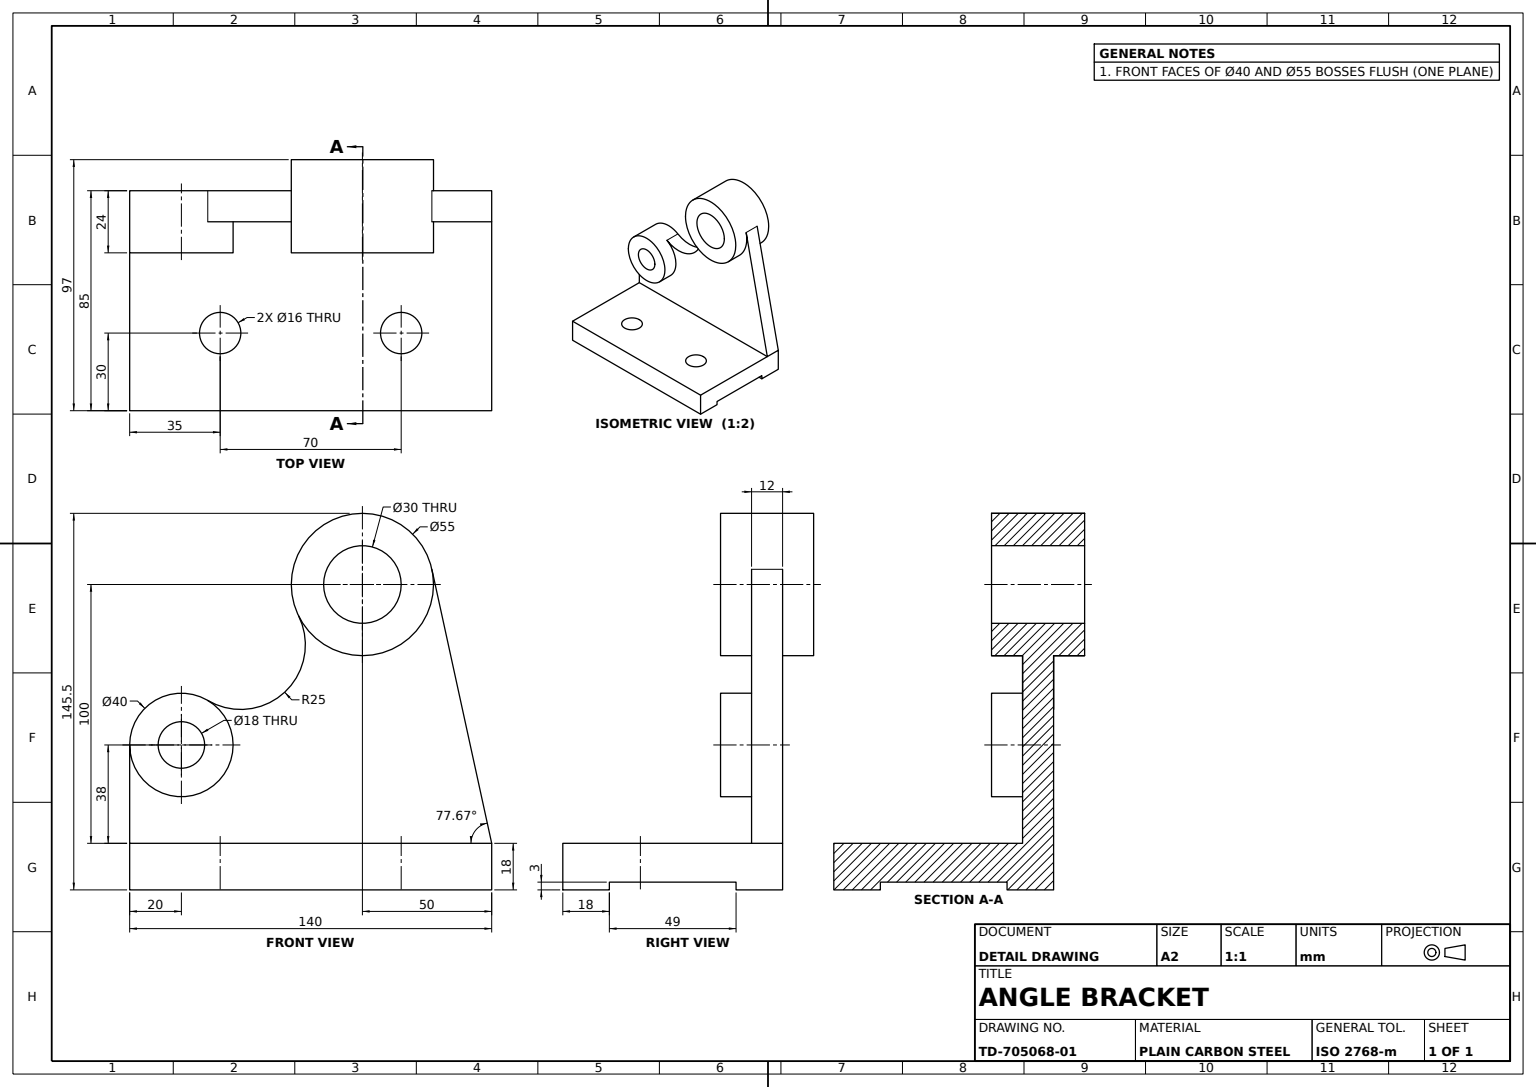
from build123d import *

# Parameters (mm, degrees)
BASE_PLATE_SKETCH_W          = 140
BASE_PLATE_SKETCH_H          = 85
BASE_PLATE_DEPTH             = 18
UNDERSIDE_GROOVE_SKETCH_W    = 49
UNDERSIDE_GROOVE_SKETCH_H    = 3
UNDERSIDE_GROOVE_DEPTH       = 148.411838059
BASE_HOLES_SKETCH_R          = 8
BASE_HOLES_DEPTH             = 84.846586096
UPRIGHT_LUG_PLATE_DEPTH      = 12
UPRIGHT_LUG_PLATE_DEPTH_BACK = 24
UPRIGHT_LUG_PLATE_SKETCH_R   = 27.5
UPRIGHT_LUG_PLATE_SKETCH_R_2 = 15
SIDE_GUSSET_SKETCH_R         = 20
SIDE_GUSSET_SKETCH_R_2       = 9
SIDE_GUSSET_DEPTH            = 24
HINGE_BOSS_EXTENSION_DEPTH   = 12


with BuildPart() as part:
    # Base Plate Sketch → Base Plate (new body)
    with BuildSketch(Plane(origin=(0, 0, 0), x_dir=(1, 0, 0), z_dir=(0, 1, 0))):
        Rectangle(BASE_PLATE_SKETCH_W, BASE_PLATE_SKETCH_H)
    extrude(amount=BASE_PLATE_DEPTH)

    # Underside Groove Sketch → Underside Groove (cut, through all)
    with BuildSketch(Plane(origin=(70, 0, 0), x_dir=(0, 0, -1), z_dir=(1, 0, 0))):
        with Locations((0, 1.5)):
            Rectangle(UNDERSIDE_GROOVE_SKETCH_W, UNDERSIDE_GROOVE_SKETCH_H)
    extrude(amount=-UNDERSIDE_GROOVE_DEPTH, mode=Mode.SUBTRACT)

    # Base Holes Sketch → Base Holes (cut, through all)
    with BuildSketch(Plane(origin=(0, 18, 0), x_dir=(1, 0, 0), z_dir=(0, 1, 0))):
        with Locations(Location((-35, -12.5, 0), (0, 0, 270))):
            Circle(BASE_HOLES_SKETCH_R)
        with Locations(Location((35, -12.5, 0), (0, 0, 270))):
            Circle(BASE_HOLES_SKETCH_R)
    extrude(amount=-BASE_HOLES_DEPTH, mode=Mode.SUBTRACT)



with BuildPart() as body_2:
    # Upright Lug Plate Sketch → Upright Lug Plate (new, two sides: drawn at the far end of the back side and taken through both)
    with BuildSketch(Plane(origin=(0, 0, -42.5), x_dir=(-1, 0, 0), z_dir=(0, 0, -1)).offset(-UPRIGHT_LUG_PLATE_DEPTH_BACK)):
        with Locations((-20, 118)):
            Circle(UPRIGHT_LUG_PLATE_SKETCH_R)
        with Locations((-20, 118)):
            Circle(UPRIGHT_LUG_PLATE_SKETCH_R_2, mode=Mode.SUBTRACT)
    extrude(amount=UPRIGHT_LUG_PLATE_DEPTH + UPRIGHT_LUG_PLATE_DEPTH_BACK)


with BuildPart() as body_3:
    # Side Gusset Sketch → Side Gusset (new body)
    with BuildSketch(Plane(origin=(0, 0, -42.5), x_dir=(-1, 0, 0), z_dir=(0, 0, -1))):
        with Locations((50, 56)):
            Circle(SIDE_GUSSET_SKETCH_R)
        with Locations((50, 56)):
            Circle(SIDE_GUSSET_SKETCH_R_2, mode=Mode.SUBTRACT)
    extrude(amount=-SIDE_GUSSET_DEPTH)


with BuildPart() as part_1:
    add(part.part)

    add(body_2.part)  # Hinge Boss Extension merges body 2

    add(body_3.part)  # Hinge Boss Extension merges body 3
    # Hinge Boss Extension Sketch → Hinge Boss Extension (add)
    with BuildSketch(Plane(origin=(0, 0, -42.5), x_dir=(-1, 0, 0), z_dir=(0, 0, -1))):
        with BuildLine():
            Line((70, 18), (70, 56))
            ThreePointArc((70, 56), (40.100426872, 38.621897345), (39.800154813, 73.203579806))
            ThreePointArc((39.800154813, 73.203579806), (10.05246179, 76.375791932), (4.645420553, 105.799457153))
            ThreePointArc((4.645420553, 105.799457153), (-29.103509689, 92.050508457), (-46.866088482, 123.870544241))
            Line((-46.866088482, 123.870544241), (-70, 18))
            Line((-70, 18), (70, 18))
        make_face()
    extrude(amount=-HINGE_BOSS_EXTENSION_DEPTH)


solid = part_1.part
